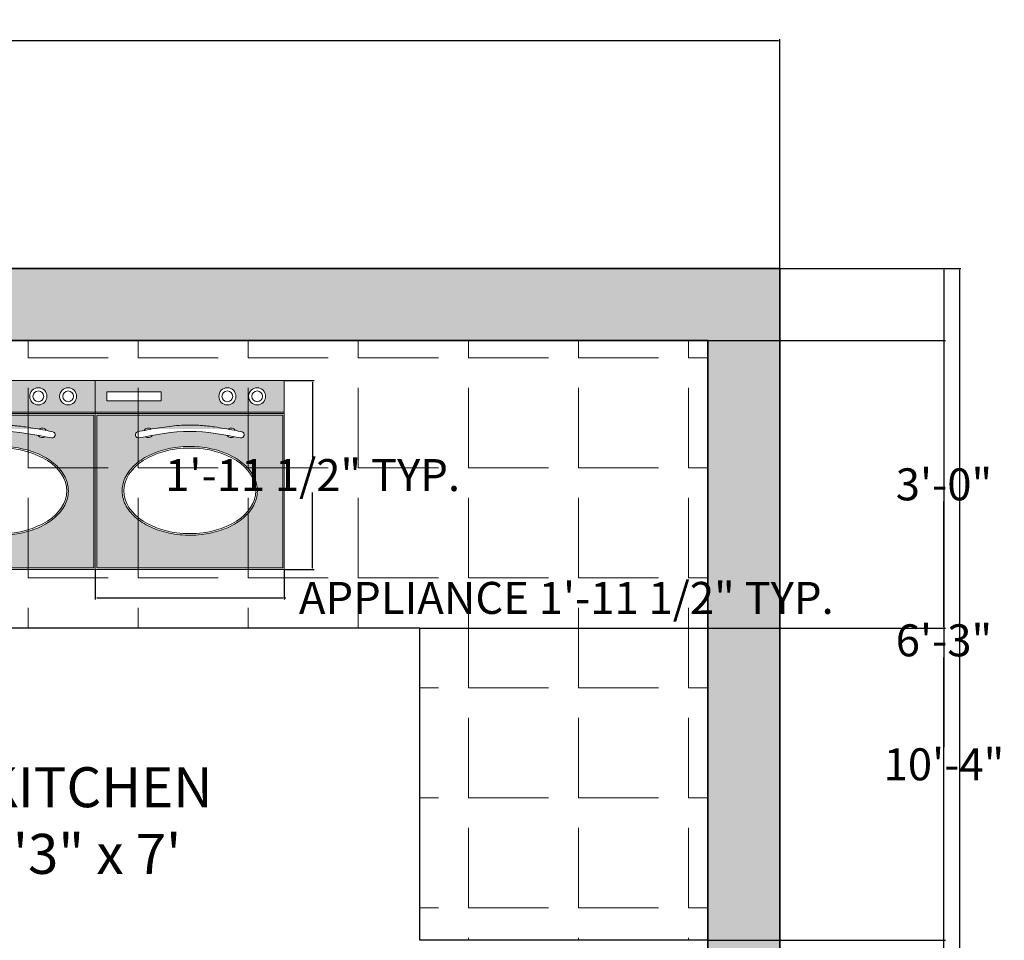
# Model space of a CAD drawing. Units: inches. Extents: x 490 to 851, y 299 to 716.
# Tile 3 of 3: x 728 to 851, y 601 to 716. Entities that reach past the tile are written whole.
import ezdxf

# ---------------------------------------------------------------- set-up
doc = ezdxf.new("R2010")
doc.units = ezdxf.units.IN
doc.header["$MEASUREMENT"] = 0
for name, color, linetype, lineweight in [('A-ANNO-DIMS', 2, 'Continuous', 18), ('A-AREA-IDEN', 7, 'Continuous', 25), ('A-EQPM', 8, 'Continuous', 18), ('A-EQPM-PATT', 9, 'Continuous', 13), ('A-FLOR-CASE', 40, 'Continuous', 25), ('A-FLOR-CASE-PATT', 9, 'Continuous', 13), ('A-WALL', 7, 'Continuous', 35), ('A-WALL-PATT', 1, 'Continuous', 13)]:
    doc.layers.add(name, color=color, linetype=linetype, lineweight=lineweight)
doc.styles.get("Standard").update_dxf_attribs({"font": 'arial.ttf'})
doc.dimstyles.get("Standard").update_dxf_attribs({"dimtxt": 4, "dimasz": 0.18, "dimexe": 0.18, "dimexo": 0.0625, "dimgap": 0.09, "dimtad": 0, "dimtih": 1, "dimtoh": 1, "dimdec": 0, "dimrnd": 6, "dimzin": 0, "dimdsep": 46, "dimlunit": 3, "dimtxsty": 'Standard', "dimcen": 0.09, "dimadec": 0, "dimazin": 0, "dimtfac": 1, "dimtdec": 0, "dimtofl": 0, "dimtmove": 0, "dimatfit": 3, "dimfxl": 1, "dimtolj": 1, "dimtzin": 0, "dimarcsym": 0})

# ---------------------------------------------------------------- blocks, each defined once
blk = doc.blocks.new('A$C7E884C79')
for p, q in [((-1.70119819813e-05, 1.5003966837e-05), (-1.70119419636e-05, 600.0000150039222)), ((-1.70119419636e-05, 600.0000150039222), (-1.70119819813e-05, 1.5003966837e-05)), ((-1.70119419636e-05, 600.0000150039222), (599.9999829879742, 600.0000150039077)), ((599.9999829879742, 600.0000150039077), (599.9999829880543, 1.5003966837e-05)), ((599.9999829880543, 1.5003966837e-05), (599.9999829879742, 600.0000150039077)), ((599.9999829879742, 600.0000150039077), (599.9999829879742, 450.0000150039659)), ((599.9999829879742, 600.0000150039077), (599.999982988058, 500.0000150039222)), ((599.999982988058, 500.0000150039222), (-1.70119383256e-05, 500.0000150039368)), ((599.999982988058, 495.0000150039441), (-1.70119019458e-05, 495.0000150039368)), ((599.999982988058, 500.0000150039222), (599.9999829880543, 1.5003966837e-05)), ((-1.70119819813e-05, 1.5003966837e-05), (599.9999829880543, 1.5003966837e-05))]:
    blk.add_line(p, q)
for points in [[(36.4219297853997, 564.739244228137), (208.9464086602384, 564.7392442281297), (208.9464086601583, 535.2607857798894), (36.4219297853997, 535.2607857798894)], [(4.999982988054398, 490.0000150040023), (594.999982988018, 490.0000150039513), (594.999982988018, 5.000015003966836), (4.999982987974362, 5.000015003930457)]]:
    blk.add_lwpolyline(points, close=True)
for centre, radius in [((419.341129777058, 550.0000150039514), 27.0465612830012), ((419.341129777058, 550.0000150039514), 17.0465612830012), ((513.9038640534054, 550.0000150040095), 27.0465612830012), ((513.9038640534054, 550.0000150040095), 17.0465612830012)]:
    blk.add_circle(centre, radius)
for centre, radius, start, end in [((168.4662399462322, 434.1738953022822), 14.99999999999999, 50.78880560725227, 150.3670062790382), ((431.5337276184946, 434.1738953023768), 14.99999999999999, 29.63299372096182, 129.2111943927477), ((137.2371143128039, 427.9571012842962), 9.99999999999936, 107.9829144627732, 276.9581094476087), ((168.4662399462322, 434.1738953022822), 14.99999999999999, 234.0164507050499, 327.1412143486447), ((431.5337276184946, 434.1738953023768), 14.99999999999999, 212.858785649389, 305.9835492949501), ((462.7628532516318, 427.957101284347), 9.99999999999936, 263.0418905523912, 72.01708553722673)]:
    blk.add_arc(centre, radius, start, end)
blk.add_ellipse((299.9999829880799, 250.0000150039296), major_axis=(-209.5453259160858, -5.8e-15), ratio=0.6483519184224599)
for points, knots in [([(134.1497789577479, 437.4685875095702), (144.6082166758169, 439.5062024863827), (155.1126203912208, 441.5529426086532), (185.9929094715517, 447.3437385568786), (206.494733029569, 450.9047119657725), (247.8674864836758, 456.3761860351832), (268.7408772092858, 458.286932131693), (293.5357101192494, 458.8504522635657), (297.2767330304487, 458.8901691064702), (304.7624299796444, 458.8727062536881), (308.4995762127364, 458.8160495901202), (319.6935092446511, 458.5127217792715), (327.132745431325, 458.1327232394569), (349.3790513168205, 456.541815341955), (364.1144689435605, 454.8805655177448), (399.790008761498, 449.8898845417889), (420.6328031065277, 446.1500348981672), (449.5099892856014, 440.6522069539087), (457.6940766911502, 439.0576405788188), (465.8501870183317, 437.4685875095119)], [0, 0, 0, 0, 31.63886493985545, 31.63886493985545, 92.6001428223882, 92.6001428223882, 153.561420704921, 153.561420704921, 164.3676472469802, 164.3676472469802, 175.1738737890395, 175.1738737890395, 196.786326873158, 196.786326873158, 240.011233041395, 240.011233041395, 302.0992006983722, 302.0992006983722, 326.7730650015291, 326.7730650015291, 326.7730650015291, 326.7730650015291]), ([(85.4546570720122, 250.000015003995), (85.45465707196854, 244.8170777658043), (85.88822561246344, 239.6342308201456), (88.02000493869853, 226.9220552357911), (90.21816192173355, 219.4365483580441), (96.38934370677816, 204.8396118246929), (100.3615888692657, 197.7281744404427), (109.949488846185, 184.0573372099134), (115.5648436689007, 177.4976038454224), (128.2787075515953, 165.0792487628459), (135.3771921305961, 159.2204529245464), (150.8720546014374, 148.3331296320939), (159.2684172301451, 143.3046103743872), (177.1485118738346, 134.1894280664528), (186.6321541176294, 130.1028504448732), (206.452394453896, 122.9637707452166), (216.7888352855625, 119.9113613978661), (238.0601333966843, 114.9105694415302), (248.9947899629697, 112.9622577759255), (271.1933164569673, 110.2148003270667), (282.4569621843111, 109.4156943254311), (305.0360465127196, 108.9852871540024), (316.3512522399324, 109.3539922337331), (338.7547296880475, 111.250649079022), (349.842772469201, 112.7785733309465), (371.5188673051307, 116.9582324470866), (382.1067079762179, 119.6099073260157), (402.521673323441, 125.9760737243086), (412.3486219806691, 129.6904786132982), (430.9992961862953, 138.0977836687561), (439.8229044345789, 142.7905902191232), (456.2471036538445, 153.0498538677457), (463.8476543751239, 158.616262825697), (477.6310685340795, 170.4997415048819), (483.8139313680366, 176.8169072710916), (494.5927765360757, 190.0604633081639), (499.1886010545786, 196.9871541335851), (506.6510537532812, 211.2839776396031), (509.5170666792983, 218.6543269104914), (513.4150547302415, 233.6388937332849), (514.4461961801352, 241.2525613148282), (514.6307693529524, 256.4928783461756), (513.7841458961847, 264.1183282945521), (510.2477897096396, 279.1482905806288), (507.5588601688614, 286.5521574531694), (500.4381704066108, 300.9341605102481), (496.0070741749878, 307.9124682590946), (485.5423204980033, 321.2743467604842), (479.5088542609591, 327.6582316730155), (466.0064121881987, 339.6881924907093), (458.5374402723464, 345.3343844510992), (442.356079099205, 355.7645443168249), (433.643722825036, 360.5484732858849), (415.1928234087136, 369.1474950443399), (405.4543904653837, 372.9624956318466), (385.1916535080673, 379.5371793190816), (374.6675208302404, 382.2967738713005), (353.0924824455687, 386.6971874674664), (342.0417855184496, 388.3379435140769), (319.6857084956864, 390.4625844960347), (308.380556257187, 390.9464386215868), (285.7940339416527, 390.7459687177425), (274.5128969021971, 390.0616475992965), (252.2522801997875, 387.5407311810659), (241.273026189534, 385.704172406523), (219.886530266871, 380.921302532438), (209.4794921704815, 377.9750595404139), (189.4937597145654, 371.0403800096638), (179.9152279588161, 367.0520348783057), (161.8232383307077, 358.1233102125143), (153.3098778178173, 353.1830191051149), (137.5613657555441, 342.4603322407738), (130.3262354594117, 336.6779568452357), (117.3219427482508, 324.3988645588861), (111.5527951950935, 317.9019950986867), (101.6427302403026, 304.3410831906103), (97.50207040229724, 297.2767107389691), (90.98281377420064, 282.7548846949166), (88.60495846102276, 275.2973569409469), (86.02335275324731, 261.8687924363285), (85.45465707200856, 255.934491795876), (85.4546570720122, 250.000015003995)], [0, 0, 0, 0, 0.1083005230516948, 0.1083005230516948, 0.2675342177864238, 0.2675342177864238, 0.4267679125211527, 0.4267679125211527, 0.5860016072558816, 0.5860016072558816, 0.7452353019906105, 0.7452353019906105, 0.9044689967253393, 0.9044689967253393, 1.063702691460068, 1.063702691460068, 1.222936386194797, 1.222936386194797, 1.382170080929526, 1.382170080929526, 1.541403775664254, 1.541403775664254, 1.700637470398983, 1.700637470398983, 1.859871165133712, 1.859871165133712, 2.019104859868441, 2.019104859868441, 2.17833855460317, 2.17833855460317, 2.337572249337898, 2.337572249337898, 2.496805944072627, 2.496805944072627, 2.656039638807356, 2.656039638807356, 2.815273333542085, 2.815273333542085, 2.974507028276814, 2.974507028276814, 3.133740723011543, 3.133740723011543, 3.292974417746271, 3.292974417746271, 3.452208112481, 3.452208112481, 3.611441807215729, 3.611441807215729, 3.770675501950458, 3.770675501950458, 3.929909196685187, 3.929909196685187, 4.089142891419916, 4.089142891419916, 4.248376586154645, 4.248376586154645, 4.407610280889374, 4.407610280889374, 4.566843975624102, 4.566843975624102, 4.726077670358831, 4.726077670358831, 4.88531136509356, 4.88531136509356, 5.044545059828289, 5.044545059828289, 5.203778754563018, 5.203778754563018, 5.363012449297746, 5.363012449297746, 5.522246144032475, 5.522246144032475, 5.681479838767204, 5.681479838767204, 5.840713533501933, 5.840713533501933, 5.999947228236662, 5.999947228236662, 6.15918092297139, 6.15918092297139, 6.283185307179586, 6.283185307179586, 6.283185307179586, 6.283185307179586])]:
    blk.add_open_spline(points, degree=3, knots=knots)
blk.add_open_spline([(137.9744605147498, 417.8376983042863), (191.9829680058602, 428.3601631990827), (299.999982988136, 449.4050929886863), (408.016997970407, 428.360163199051), (462.0255054615699, 417.837698304228)], degree=3)
blk = doc.blocks.new('*D102')
at = {"layer": 'A-ANNO-DIMS', "color": 0, "lineweight": -2, "transparency": 16777216}
for p, q in [((546.6878542437281, 685.0194991519433), (546.6878542437281, 713.5977998437985)), ((546.867854243728, 713.4177998437985), (681.1694777089394, 713.4177998437985)), ((822.507854243728, 713.4177998437985), (688.2062307785166, 713.4177998437985)), ((822.687854243728, 685.0194991519433), (822.687854243728, 713.5977998437985))]:
    blk.add_line(p, q, dxfattribs=at)
at = {"layer": 'A-ANNO-DIMS', "color": 0, "transparency": 16777216}
for points in [[(546.867854243728, 713.4477998437985), (546.867854243728, 713.3877998437985), (546.6878542437281, 713.4177998437985)], [(822.507854243728, 713.4477998437985), (822.507854243728, 713.3877998437985), (822.687854243728, 713.4177998437985)]]:
    blk.add_solid(points, dxfattribs=at)
at = {"layer": 'Defpoints', "color": 0, "transparency": 16777216}
for p in [(822.687854243728, 713.4177998437985), (546.6878542437281, 684.9569991519433), (822.687854243728, 684.9569991519433)]:
    blk.add_point(p, dxfattribs=at)
at = {"layer": 'A-ANNO-DIMS', "color": 0, "transparency": 16777216, "insert": (684.687854243728, 713.4177998437985), "char_height": 4, "attachment_point": 5}
blk.add_mtext("\\A1;23'", dxfattribs=at)
blk = doc.blocks.new('*D103')
at = {"layer": 'A-ANNO-DIMS', "color": 0, "lineweight": -2, "transparency": 16777216}
for p, q in [((822.7503542437285, 684.9569991519436), (845.3273379142681, 684.9569991519436)), ((845.147337914268, 684.7769991519436), (845.147337914268, 507.0906553593105)), ((845.147337914268, 325.1369991519435), (845.147337914268, 502.8233429445765)), ((822.7503542437283, 324.9569991519435), (845.3273379142681, 324.9569991519435))]:
    blk.add_line(p, q, dxfattribs=at)
at = {"layer": 'A-ANNO-DIMS', "color": 0, "transparency": 16777216}
for points in [[(845.117337914268, 684.7769991519436), (845.1773379142682, 684.7769991519436), (845.147337914268, 684.9569991519436)], [(845.117337914268, 325.1369991519435), (845.1773379142682, 325.1369991519435), (845.147337914268, 324.9569991519435)]]:
    blk.add_solid(points, dxfattribs=at)
at = {"layer": 'Defpoints', "color": 0, "transparency": 16777216}
for p in [(822.6878542437285, 684.9569991519436), (822.6878542437283, 324.9569991519435), (845.147337914268, 324.9569991519435)]:
    blk.add_point(p, dxfattribs=at)
at = {"layer": 'A-ANNO-DIMS', "color": 0, "transparency": 16777216, "insert": (845.147337914268, 504.9569991519431), "char_height": 4, "attachment_point": 5}
blk.add_mtext("\\A1;30'", dxfattribs=at)
blk = doc.blocks.new('*D114')
at = {"layer": 'A-ANNO-DIMS', "color": 0, "lineweight": -2, "transparency": 16777216}
for p, q in [((737.131587064389, 647.2418630191439), (737.131587064389, 643.5810559325296)), ((760.753634308485, 647.2418630191439), (760.753634308485, 643.5810559325296)), ((737.3115870643888, 643.7610559325295), (760.5736343084851, 643.7610559325295)), ((760.753634308485, 643.7610559325295), (760.933634308485, 643.7610559325295))]:
    blk.add_line(p, q, dxfattribs=at)
at = {"layer": 'A-ANNO-DIMS', "color": 0, "transparency": 16777216}
for points in [[(737.3115870643888, 643.7910559325294), (737.3115870643888, 643.7310559325294), (737.131587064389, 643.7610559325295)], [(760.5736343084851, 643.7910559325294), (760.5736343084851, 643.7310559325294), (760.753634308485, 643.7610559325295)]]:
    blk.add_solid(points, dxfattribs=at)
at = {"layer": 'Defpoints', "color": 0, "transparency": 16777216}
for p in [(737.131587064389, 647.3043630191439), (760.753634308485, 647.3043630191439), (760.753634308485, 643.7610559325295)]:
    blk.add_point(p, dxfattribs=at)
at = {"layer": 'A-ANNO-DIMS', "color": 0, "transparency": 16777216, "insert": (796.004534717762, 643.7610559325295), "char_height": 4, "attachment_point": 5}
blk.add_mtext('\\A1;APPLIANCE 1\'-11 1/2" TYP.', dxfattribs=at)
blk = doc.blocks.new('*D115')
at = {"layer": 'A-ANNO-DIMS', "color": 0, "lineweight": -2, "transparency": 16777216}
for p, q in [((760.8161343084852, 670.9264102632369), (764.4769413950997, 670.9264102632369)), ((764.2969413950999, 670.746410263237), (764.2969413950999, 661.2735994652013)), ((764.2969413950999, 647.4843630191441), (764.2969413950999, 656.9571738171796)), ((760.8161343084852, 647.3043630191441), (764.4769413950997, 647.3043630191441))]:
    blk.add_line(p, q, dxfattribs=at)
at = {"layer": 'A-ANNO-DIMS', "color": 0, "transparency": 16777216}
for points in [[(764.2669413950999, 670.746410263237), (764.3269413950998, 670.746410263237), (764.2969413950999, 670.9264102632369)], [(764.2669413950999, 647.4843630191441), (764.3269413950998, 647.4843630191441), (764.2969413950999, 647.3043630191441)]]:
    blk.add_solid(points, dxfattribs=at)
at = {"layer": 'Defpoints', "color": 0, "transparency": 16777216}
for p in [(760.7536343084852, 670.9264102632369), (764.2969413950999, 670.9264102632369), (760.7536343084852, 647.3043630191441)]:
    blk.add_point(p, dxfattribs=at)
at = {"layer": 'A-ANNO-DIMS', "color": 0, "transparency": 16777216, "insert": (764.2969413950999, 659.1153866411903), "char_height": 4, "attachment_point": 5}
blk.add_mtext('\\A1;1\'-11 1/2" TYP.', dxfattribs=at)
blk = doc.blocks.new('*D139')
at = {"layer": 'A-ANNO-DIMS', "color": 0, "lineweight": -2, "transparency": 16777216}
for p, q in [((813.7503540000004, 675.9569990000002), (843.3817780000008, 675.9569990000002)), ((843.2017780000009, 675.7769990000002), (843.2017780000009, 660.0906552073673)), ((843.2017780000009, 640.1369990000001), (843.2017780000009, 655.8233427926332)), ((777.7503540000004, 639.9569990000002), (843.3817780000008, 639.9569990000002))]:
    blk.add_line(p, q, dxfattribs=at)
at = {"layer": 'A-ANNO-DIMS', "color": 0, "transparency": 16777216}
for points in [[(843.171778000001, 675.7769990000002), (843.2317780000008, 675.7769990000002), (843.2017780000009, 675.9569990000002)], [(843.171778000001, 640.1369990000001), (843.2317780000008, 640.1369990000001), (843.2017780000009, 639.9569990000002)]]:
    blk.add_solid(points, dxfattribs=at)
at = {"layer": 'Defpoints', "color": 0, "transparency": 16777216}
for p in [(813.6878540000004, 675.9569990000002), (843.2017780000009, 675.9569990000002), (777.6878540000004, 639.9569990000002)]:
    blk.add_point(p, dxfattribs=at)
at = {"layer": 'A-ANNO-DIMS', "color": 0, "transparency": 16777216, "insert": (843.2017780000007, 657.9569989999998), "char_height": 4, "attachment_point": 5}
blk.add_mtext('\\A1;3\'-0"', dxfattribs=at)
blk = doc.blocks.new('*D140')
at = {"layer": 'A-ANNO-DIMS', "color": 0, "lineweight": -2, "transparency": 16777216}
for p, q in [((813.7503540000004, 675.9569990000002), (843.3817780000008, 675.9569990000002)), ((843.2017780000009, 675.7769990000002), (843.2017780000009, 640.5906552073671)), ((843.2017780000009, 601.1369990000002), (843.2017780000009, 636.3233427926331)), ((813.7503540000004, 600.9569990000002), (843.3817780000008, 600.9569990000002))]:
    blk.add_line(p, q, dxfattribs=at)
at = {"layer": 'A-ANNO-DIMS', "color": 0, "transparency": 16777216}
for points in [[(843.171778000001, 675.7769990000002), (843.2317780000008, 675.7769990000002), (843.2017780000009, 675.9569990000002)], [(843.171778000001, 601.1369990000002), (843.2317780000008, 601.1369990000002), (843.2017780000009, 600.9569990000002)]]:
    blk.add_solid(points, dxfattribs=at)
at = {"layer": 'Defpoints', "color": 0, "transparency": 16777216}
for p in [(813.6878540000004, 675.9569990000002), (843.2017780000009, 675.9569990000002), (813.6878540000004, 600.9569990000002)]:
    blk.add_point(p, dxfattribs=at)
at = {"layer": 'A-ANNO-DIMS', "color": 0, "transparency": 16777216, "insert": (843.2017780000007, 638.4569989999999), "char_height": 4, "attachment_point": 5}
blk.add_mtext('\\A1;6\'-3"', dxfattribs=at)
blk = doc.blocks.new('*D142')
at = {"layer": 'A-ANNO-DIMS', "color": 0, "lineweight": -2, "transparency": 16777216}
for p, q in [((822.7503540000004, 684.9569990000002), (843.3817780000008, 684.9569990000002)), ((843.2017780000009, 684.7769990000003), (843.2017780000009, 625.089290950887)), ((843.2017780000009, 561.1369990000001), (843.2017780000009, 620.8247070491134)), ((813.7503540000004, 560.9569990000002), (843.3817780000008, 560.9569990000002))]:
    blk.add_line(p, q, dxfattribs=at)
at = {"layer": 'A-ANNO-DIMS', "color": 0, "transparency": 16777216}
for points in [[(843.171778000001, 684.7769990000003), (843.2317780000008, 684.7769990000003), (843.2017780000009, 684.9569990000002)], [(843.171778000001, 561.1369990000001), (843.2317780000008, 561.1369990000001), (843.2017780000009, 560.9569990000002)]]:
    blk.add_solid(points, dxfattribs=at)
at = {"layer": 'Defpoints', "color": 0, "transparency": 16777216}
for p in [(822.6878540000004, 684.9569990000002), (843.2017780000009, 684.9569990000002), (813.6878540000004, 560.9569990000002)]:
    blk.add_point(p, dxfattribs=at)
at = {"layer": 'A-ANNO-DIMS', "color": 0, "transparency": 16777216, "insert": (843.2017780000007, 622.9569989999999), "char_height": 4, "attachment_point": 5}
blk.add_mtext('\\A1;10\'-4"', dxfattribs=at)

msp = doc.modelspace()

# ---------------------------------------------------------------- hatches: boundary and pattern name
at = {"layer": 'A-EQPM-PATT'}
h = msp.add_hatch(color=256, dxfattribs=at)
h.dxf.hatch_style = 1
edge = h.paths.add_edge_path(flags=0)
edge.add_ellipse((725.3205634423474, 657.1468827041818), major_axis=(8.249815980948258, 3.137e-13), ratio=0.648351918422466, start_angle=0, end_angle=360)
edge = h.paths.add_edge_path(flags=0)
edge.add_ellipse((748.9426106864386, 657.1468827041818), major_axis=(8.249815980948258, 3.137e-13), ratio=0.648351918422466, start_angle=0, end_angle=360)
h.paths.add_polyline_path([(760.5567839147827, 666.5957016018205), (737.3284374580912, 666.5957016018225), (737.328437458088, 647.5012134128433), (760.5567839147827, 647.5012134128445)])
edge = h.paths.add_edge_path(flags=16)
edge.add_spline(control_points=[(740.4959443117903, 657.1468827041843), (740.4959443117887, 656.9428300570115), (740.513013939367, 656.7387809646627), (740.5969422592976, 656.238301610948), (740.683483872803, 655.943596615761), (740.9264437855999, 655.368914075078), (741.0828313904223, 655.0889362253043), (741.4603077674664, 654.5507142870945), (741.6813847289907, 654.2924570680201), (742.181930551144, 653.8035454505958), (742.461398447955, 653.5728841971194), (743.0714324035, 653.1442494218261), (743.4019978613231, 652.9462762227037), (744.1059385953266, 652.5874107775095), (744.4793103372083, 652.4265218947702), (745.259634759896, 652.1454557648624), (745.6665812493317, 652.0252821685099), (746.5040339308719, 651.8284005954259), (746.934532220883, 651.7516954117406), (747.8084899568673, 651.6435277956438), (748.251940576054, 651.6120669294378), (749.1408809039442, 651.5951217652083), (749.5863614443855, 651.6096377132291), (750.4683881155711, 651.6843092425713), (750.9049252329394, 651.7444637406785), (751.758314793409, 651.9090172491879), (752.1751589143181, 652.0134138979646), (752.9788977075159, 652.2640503703385), (753.3657854499264, 652.4102867832906), (754.1000639619589, 652.7412830453165), (754.4474501134661, 652.926039208717), (755.0940721299727, 653.3299472263792), (755.393306410338, 653.5490971853537), (755.9359605110842, 654.0169506766601), (756.1793803076966, 654.2656579902905), (756.6037442906904, 654.7870578342696), (756.7846822638598, 655.0597621974754), (757.0784796142024, 655.6226292646414), (757.1913147687701, 655.9128004957787), (757.344778865264, 656.5027440714792), (757.3853749853384, 656.802494763666), (757.3926416456854, 657.4025072452151), (757.3593100135294, 657.7027218101118), (757.2200833920119, 658.2944526087763), (757.1142200242647, 658.5859434305298), (756.8338779076405, 659.152164023328), (756.6594253000964, 659.4269005488733), (756.2474271238373, 659.9529587575895), (756.0098890830087, 660.204292809264), (755.4782968754197, 660.6779133138975), (755.1842428629845, 660.9002043359601), (754.5471813994751, 661.310840551146), (754.2041752469486, 661.4991842113454), (753.4777618841014, 661.8377283750641), (753.0943590123167, 661.987925248588), (752.2966134628161, 662.246771063046), (751.8822775306182, 662.3554165178577), (751.0328665705918, 662.5286611476281), (750.5977997624374, 662.5932578423766), (749.7176392497302, 662.6769051251308), (749.2725545159311, 662.6959545001525), (748.3833213539021, 662.6880619842531), (747.9391821003803, 662.6611202079364), (747.0627798680019, 662.5618715300532), (746.63052577311, 662.4895660664885), (745.7885377446587, 662.3012641029419), (745.378811835352, 662.1852702843584), (744.591971974883, 661.912251405195), (744.214864425444, 661.7552299433305), (743.5025813692192, 661.403705350189), (743.1674096954835, 661.2092057002914), (742.5473895355515, 660.7870526741362), (742.2625418860974, 660.5594000995088), (741.750561858099, 660.0759712693376), (741.5234300646675, 659.820189007125), (741.1332700270774, 659.2862948375157), (740.9702519232188, 659.0081699378447), (740.7135882764434, 658.4364445030395), (740.6199719255308, 658.1428410481587), (740.5183339055397, 657.6141574062448), (740.4959443117901, 657.3805235227624), (740.4959443117903, 657.1468827041843)], knot_values=[0, 0, 0, 0, 0.1083005230516948, 0.1083005230516948, 0.2675342177864238, 0.2675342177864238, 0.4267679125211527, 0.4267679125211527, 0.5860016072558816, 0.5860016072558816, 0.7452353019906105, 0.7452353019906105, 0.9044689967253393, 0.9044689967253393, 1.063702691460068, 1.063702691460068, 1.222936386194797, 1.222936386194797, 1.382170080929526, 1.382170080929526, 1.541403775664254, 1.541403775664254, 1.700637470398983, 1.700637470398983, 1.859871165133712, 1.859871165133712, 2.019104859868441, 2.019104859868441, 2.17833855460317, 2.17833855460317, 2.337572249337898, 2.337572249337898, 2.496805944072627, 2.496805944072627, 2.656039638807356, 2.656039638807356, 2.815273333542085, 2.815273333542085, 2.974507028276814, 2.974507028276814, 3.133740723011543, 3.133740723011543, 3.292974417746271, 3.292974417746271, 3.452208112481, 3.452208112481, 3.611441807215729, 3.611441807215729, 3.770675501950458, 3.770675501950458, 3.929909196685187, 3.929909196685187, 4.089142891419916, 4.089142891419916, 4.248376586154645, 4.248376586154645, 4.407610280889374, 4.407610280889374, 4.566843975624102, 4.566843975624102, 4.726077670358831, 4.726077670358831, 4.88531136509356, 4.88531136509356, 5.044545059828289, 5.044545059828289, 5.203778754563018, 5.203778754563018, 5.363012449297746, 5.363012449297746, 5.522246144032475, 5.522246144032475, 5.681479838767204, 5.681479838767204, 5.840713533501933, 5.840713533501933, 5.999947228236662, 5.999947228236662, 6.15918092297139, 6.15918092297139, 6.283185307179586, 6.283185307179586, 6.283185307179586, 6.283185307179586], degree=3, periodic=0)
edge = h.paths.add_edge_path(flags=0)
edge.add_ellipse((748.9426106864386, 657.1468827041818), major_axis=(8.249815980948258, 3.137e-13), ratio=0.648351918422466, start_angle=0, end_angle=360)
edge = h.paths.add_edge_path(flags=16)
edge.add_spline(control_points=[(742.4130750946933, 664.5275351650338), (742.6914882918603, 664.5817783431816), (742.9707288907302, 664.6361857766777), (743.2508036674241, 664.6898164654069)], knot_values=[0, 0, 0, 0, 21.39329177210675, 21.39329177210675, 21.39329177210675, 21.39329177210675], degree=3, periodic=0)
edge.add_arc((743.7641168658934, 664.3978228734082), 0.5905511811023694, 50.78880560234279, 150.3670062825767, ccw=False)
edge.add_spline(control_points=[(744.1374519240431, 664.8553943233596), (744.779067646516, 664.97139206178), (745.4250780596886, 665.0781755879807), (746.8901501941393, 665.2719288077744), (747.7119372305805, 665.3471550320465), (748.688111754595, 665.36934086401), (748.8353961211775, 665.3709045192425), (749.1301085994924, 665.3702170053534), (749.2772403409527, 665.3679864280476), (749.7179463658312, 665.3560443882504), (750.0108296802672, 665.3410838158167), (750.8866684946568, 665.2784496466238), (751.4668030468905, 665.2130461102375), (752.8713518586205, 665.0165626072471), (753.6919343131492, 664.8693244323014), (754.8288314068135, 664.6528745132362), (755.1510395723863, 664.5900963094923), (755.4721462781808, 664.5275351650314)], knot_values=[43.89785635095746, 43.89785635095746, 43.89785635095746, 43.89785635095746, 92.6001428223882, 92.6001428223882, 153.561420704921, 153.561420704921, 164.3676472469802, 164.3676472469802, 175.1738737890395, 175.1738737890395, 196.786326873158, 196.786326873158, 240.011233041395, 240.011233041395, 302.0992006983722, 302.0992006983722, 326.7730650015291, 326.7730650015291, 326.7730650015291, 326.7730650015291], degree=3, periodic=0)
edge.add_arc((754.1211045695258, 664.397822873412), 0.5905511811023695, 29.64555569566221, 129.3131094229314, ccw=False)
edge.add_spline(control_points=[(744.1374519240431, 664.8553943233596), (744.779067646516, 664.97139206178), (745.4250780596886, 665.0781755879807), (746.8901501941393, 665.2719288077744), (747.7119372305805, 665.3471550320465), (748.688111754595, 665.36934086401), (748.8353961211775, 665.3709045192425), (749.1301085994924, 665.3702170053534), (749.2772403409527, 665.3679864280476), (749.7179463658312, 665.3560443882504), (750.0108296802672, 665.3410838158167), (750.8866684946568, 665.2784496466238), (751.4668030468905, 665.2130461102375), (752.8713518586205, 665.0165626072471), (753.6919343131492, 664.8693244323014), (754.8288314068135, 664.6528745132362), (755.1510395723863, 664.5900963094923), (755.4721462781808, 664.5275351650314)], knot_values=[43.89785635095746, 43.89785635095746, 43.89785635095746, 43.89785635095746, 92.6001428223882, 92.6001428223882, 153.561420704921, 153.561420704921, 164.3676472469802, 164.3676472469802, 175.1738737890395, 175.1738737890395, 196.786326873158, 196.786326873158, 240.011233041395, 240.011233041395, 302.0992006983722, 302.0992006983722, 326.7730650015291, 326.7730650015291, 326.7730650015291, 326.7730650015291], degree=3, periodic=0)
edge.add_arc((755.3505977046888, 664.1530672034108), 0.3937007874015679, -101.0087676412142, 72.01708553236932, ccw=False)
edge.add_spline(control_points=[(755.3215682641351, 663.7546655112802), (755.037073723253, 663.810093516205), (754.7525791823709, 663.8655215211298), (754.4680846414888, 663.9199572781217)], knot_values=[304.9124823041715, 304.9124823041715, 304.9124823041715, 304.9124823041715, 326.7730650015789, 326.7730650015789, 326.7730650015789, 326.7730650015789], degree=3, periodic=0)
edge.add_arc((754.1211045695258, 664.397822873412), 0.5905511811023683, 212.8587871331284, 305.9835477310444, ccw=False)
edge.add_spline(control_points=[(753.6250354635439, 664.0774073001456), (752.0642272045088, 664.3599897262603), (748.9426107100477, 664.8064223787223), (745.8209942155868, 664.3599897330135), (744.2601859801605, 664.0774073129695)], knot_values=[43.45390602737222, 43.45390602737222, 43.45390602737222, 43.45390602737222, 163.3865343148396, 283.3191607881738, 283.3191607881738, 283.3191607881738, 283.3191607881738], degree=3, periodic=0)
edge.add_arc((743.7641168658934, 664.3978228734082), 0.5905511811023553, 234.01645070441748, 327.1412143484826, ccw=False)
edge.add_spline(control_points=[(743.417136780882, 663.9199572875928), (743.1326422235041, 663.8655215275596), (742.8481476661264, 663.8100935194209), (742.5636531087486, 663.7546655112824)], knot_values=[0, 0, 0, 0, 21.86058396493695, 21.86058396493695, 21.86058396493695, 21.86058396493695], degree=3, periodic=0)
edge.add_arc((742.5346237307191, 664.1530672034088), 0.393700787401568, 107.9829001472302, 281.00876763934195, ccw=False)
h.paths.add_polyline_path([(736.9347366706914, 666.5957016018205), (713.706390214, 666.5957016018225), (713.7063902139969, 647.5012134128433), (736.9347366706914, 647.5012134128445)])
edge = h.paths.add_edge_path(flags=16)
edge.add_spline(control_points=[(716.8738970676992, 657.1468827041843), (716.8738970676975, 656.9428300570115), (716.8909666952759, 656.7387809646627), (716.9748950152064, 656.238301610948), (717.0614366287118, 655.943596615761), (717.3043965415088, 655.368914075078), (717.4607841463312, 655.0889362253043), (717.8382605233752, 654.5507142870945), (718.0593374848995, 654.2924570680201), (718.5598833070528, 653.8035454505958), (718.8393512038638, 653.5728841971194), (719.4493851594088, 653.1442494218261), (719.7799506172319, 652.9462762227037), (720.4838913512355, 652.5874107775095), (720.8572630931171, 652.4265218947702), (721.6375875158049, 652.1454557648624), (722.0445340052405, 652.0252821685099), (722.8819866867807, 651.8284005954259), (723.312484976792, 651.7516954117406), (724.1864427127762, 651.6435277956438), (724.6298933319629, 651.6120669294378), (725.518833659853, 651.5951217652083), (725.9643142002944, 651.6096377132291), (726.84634087148, 651.6843092425713), (727.2828779888483, 651.7444637406785), (728.136267549318, 651.9090172491879), (728.5531116702269, 652.0134138979646), (729.3568504634247, 652.2640503703385), (729.7437382058351, 652.4102867832906), (730.4780167178678, 652.7412830453165), (730.825402869375, 652.926039208717), (731.4720248858815, 653.3299472263792), (731.7712591662468, 653.5490971853537), (732.3139132669932, 654.0169506766601), (732.5573330636055, 654.2656579902905), (732.9816970465993, 654.7870578342696), (733.1626350197686, 655.0597621974754), (733.4564323701113, 655.6226292646414), (733.5692675246789, 655.9128004957787), (733.7227316211728, 656.5027440714792), (733.7633277412472, 656.802494763666), (733.7705944015944, 657.4025072452151), (733.7372627694382, 657.7027218101118), (733.5980361479207, 658.2944526087763), (733.4921727801734, 658.5859434305298), (733.2118306635494, 659.152164023328), (733.0373780560052, 659.4269005488733), (732.6253798797461, 659.9529587575895), (732.3878418389176, 660.204292809264), (731.8562496313285, 660.6779133138975), (731.5621956188934, 660.9002043359601), (730.925134155384, 661.310840551146), (730.5821280028575, 661.4991842113454), (729.8557146400102, 661.8377283750641), (729.4723117682256, 661.987925248588), (728.6745662187249, 662.246771063046), (728.2602302865271, 662.3554165178577), (727.4108193265005, 662.5286611476281), (726.9757525183463, 662.5932578423766), (726.0955920056391, 662.6769051251308), (725.65050727184, 662.6959545001525), (724.761274109811, 662.6880619842531), (724.317134856289, 662.6611202079364), (723.4407326239107, 662.5618715300532), (723.0084785290189, 662.4895660664885), (722.1664905005676, 662.3012641029419), (721.7567645912609, 662.1852702843584), (720.9699247307918, 661.912251405195), (720.5928171813528, 661.7552299433305), (719.880534125128, 661.403705350189), (719.5453624513922, 661.2092057002914), (718.9253422914603, 660.7870526741362), (718.6404946420062, 660.5594000995088), (718.1285146140078, 660.0759712693376), (717.9013828205763, 659.820189007125), (717.5112227829862, 659.2862948375157), (717.3482046791275, 659.0081699378447), (717.0915410323522, 658.4364445030395), (716.9979246814397, 658.1428410481587), (716.8962866614485, 657.6141574062448), (716.8738970676989, 657.3805235227624), (716.8738970676992, 657.1468827041843)], knot_values=[0, 0, 0, 0, 0.1083005230516948, 0.1083005230516948, 0.2675342177864238, 0.2675342177864238, 0.4267679125211527, 0.4267679125211527, 0.5860016072558816, 0.5860016072558816, 0.7452353019906105, 0.7452353019906105, 0.9044689967253393, 0.9044689967253393, 1.063702691460068, 1.063702691460068, 1.222936386194797, 1.222936386194797, 1.382170080929526, 1.382170080929526, 1.541403775664254, 1.541403775664254, 1.700637470398983, 1.700637470398983, 1.859871165133712, 1.859871165133712, 2.019104859868441, 2.019104859868441, 2.17833855460317, 2.17833855460317, 2.337572249337898, 2.337572249337898, 2.496805944072627, 2.496805944072627, 2.656039638807356, 2.656039638807356, 2.815273333542085, 2.815273333542085, 2.974507028276814, 2.974507028276814, 3.133740723011543, 3.133740723011543, 3.292974417746271, 3.292974417746271, 3.452208112481, 3.452208112481, 3.611441807215729, 3.611441807215729, 3.770675501950458, 3.770675501950458, 3.929909196685187, 3.929909196685187, 4.089142891419916, 4.089142891419916, 4.248376586154645, 4.248376586154645, 4.407610280889374, 4.407610280889374, 4.566843975624102, 4.566843975624102, 4.726077670358831, 4.726077670358831, 4.88531136509356, 4.88531136509356, 5.044545059828289, 5.044545059828289, 5.203778754563018, 5.203778754563018, 5.363012449297746, 5.363012449297746, 5.522246144032475, 5.522246144032475, 5.681479838767204, 5.681479838767204, 5.840713533501933, 5.840713533501933, 5.999947228236662, 5.999947228236662, 6.15918092297139, 6.15918092297139, 6.283185307179586, 6.283185307179586, 6.283185307179586, 6.283185307179586], degree=3, periodic=0)
edge = h.paths.add_edge_path(flags=0)
edge.add_ellipse((725.3205634423474, 657.1468827041818), major_axis=(8.249815980948258, 3.137e-13), ratio=0.648351918422466, start_angle=0, end_angle=360)
edge = h.paths.add_edge_path(flags=16)
edge.add_spline(control_points=[(731.6995210200438, 663.7546655112802), (731.4150264791617, 663.810093516205), (731.1305319382795, 663.8655215211298), (730.8460373973976, 663.9199572781217)], knot_values=[304.9124823041715, 304.9124823041715, 304.9124823041715, 304.9124823041715, 326.7730650015789, 326.7730650015789, 326.7730650015789, 326.7730650015789], degree=3, periodic=0)
edge.add_arc((730.4990573254347, 664.397822873412), 0.5905511811023683, 212.8587871331377, 305.9835477310444, ccw=False)
edge.add_spline(control_points=[(730.0029882194526, 664.0774073001456), (728.4421799604175, 664.3599897262603), (725.3205634659566, 664.8064223787223), (722.1989469714956, 664.3599897330135), (720.6381387360695, 664.0774073129695)], knot_values=[43.45390602737222, 43.45390602737222, 43.45390602737222, 43.45390602737222, 163.3865343148396, 283.3191607881738, 283.3191607881738, 283.3191607881738, 283.3191607881738], degree=3, periodic=0)
edge.add_arc((720.1420696218023, 664.3978228734082), 0.5905511811023554, 234.01645070441748, 327.14121434847334, ccw=False)
edge.add_spline(control_points=[(719.7950895367909, 663.9199572875928), (719.5105949794131, 663.8655215275596), (719.2261004220353, 663.8100935194209), (718.9416058646574, 663.7546655112824)], knot_values=[0, 0, 0, 0, 21.86058396493695, 21.86058396493695, 21.86058396493695, 21.86058396493695], degree=3, periodic=0)
edge.add_arc((718.9125764866279, 664.1530672034088), 0.393700787401568, 107.9829001472302, 281.00876763934195, ccw=False)
edge.add_spline(control_points=[(718.7910278506022, 664.5275351650338), (719.0694410477691, 664.5817783431816), (719.3486816466392, 664.6361857766777), (719.628756423333, 664.6898164654069)], knot_values=[0, 0, 0, 0, 21.39329177210675, 21.39329177210675, 21.39329177210675, 21.39329177210675], degree=3, periodic=0)
edge.add_arc((720.1420696218023, 664.3978228734082), 0.5905511811023695, 50.78880560234978, 150.3670062825767, ccw=False)
edge.add_spline(control_points=[(720.5154046799519, 664.8553943233596), (721.1570204024248, 664.97139206178), (721.8030308155975, 665.0781755879807), (723.268102950048, 665.2719288077744), (724.0898899864894, 665.3471550320465), (725.0660645105037, 665.36934086401), (725.2133488770864, 665.3709045192425), (725.5080613554012, 665.3702170053534), (725.6551930968615, 665.3679864280476), (726.0958991217401, 665.3560443882504), (726.388782436176, 665.3410838158167), (727.2646212505655, 665.2784496466238), (727.8447558027995, 665.2130461102375), (729.2493046145294, 665.0165626072471), (730.069887069058, 664.8693244323014), (731.2067841627223, 664.6528745132362), (731.5289923282951, 664.5900963094923), (731.8500990340896, 664.5275351650314)], knot_values=[43.89785635095746, 43.89785635095746, 43.89785635095746, 43.89785635095746, 92.6001428223882, 92.6001428223882, 153.561420704921, 153.561420704921, 164.3676472469802, 164.3676472469802, 175.1738737890395, 175.1738737890395, 196.786326873158, 196.786326873158, 240.011233041395, 240.011233041395, 302.0992006983722, 302.0992006983722, 326.7730650015291, 326.7730650015291, 326.7730650015291, 326.7730650015291], degree=3, periodic=0)
edge.add_arc((730.4990573254347, 664.397822873412), 0.5905511811023695, 29.64555569566221, 129.3131094229314, ccw=False)
edge.add_spline(control_points=[(720.5154046799519, 664.8553943233596), (721.1570204024248, 664.97139206178), (721.8030308155975, 665.0781755879807), (723.268102950048, 665.2719288077744), (724.0898899864894, 665.3471550320465), (725.0660645105037, 665.36934086401), (725.2133488770864, 665.3709045192425), (725.5080613554012, 665.3702170053534), (725.6551930968615, 665.3679864280476), (726.0958991217401, 665.3560443882504), (726.388782436176, 665.3410838158167), (727.2646212505655, 665.2784496466238), (727.8447558027995, 665.2130461102375), (729.2493046145294, 665.0165626072471), (730.069887069058, 664.8693244323014), (731.2067841627223, 664.6528745132362), (731.5289923282951, 664.5900963094923), (731.8500990340896, 664.5275351650314)], knot_values=[43.89785635095746, 43.89785635095746, 43.89785635095746, 43.89785635095746, 92.6001428223882, 92.6001428223882, 153.561420704921, 153.561420704921, 164.3676472469802, 164.3676472469802, 175.1738737890395, 175.1738737890395, 196.786326873158, 196.786326873158, 240.011233041395, 240.011233041395, 302.0992006983722, 302.0992006983722, 326.7730650015291, 326.7730650015291, 326.7730650015291, 326.7730650015291], degree=3, periodic=0)
edge.add_arc((731.7285504605976, 664.1530672034108), 0.393700787401568, -101.0087676412142, 72.01708553236932, ccw=False)
h.paths.add_polyline_path([(737.1315870643906, 670.9264102632361), (713.5095398202994, 670.9264102632366), (713.5095398202992, 666.9894023892214), (737.131587064391, 666.9894023892209)])
h.paths.add_polyline_path([(728.954208541008, 668.9579063262299, -1), (731.0838590357325, 668.9579063262299, -1)], flags=16)
h.paths.add_polyline_path([(729.3479093284096, 668.9579063262299, -1), (730.6901582483309, 668.9579063262299, -1)], flags=0)
h.paths.add_polyline_path([(721.7357770514844, 668.3776217111093), (714.9434747335805, 668.3776217111093), (714.9434747335805, 669.5381909413553), (721.7357770514876, 669.538190941355)], flags=16)
h.paths.add_polyline_path([(732.6771508353524, 668.9579063262321, -1), (734.806801330077, 668.9579063262321, -1)], flags=16)
h.paths.add_polyline_path([(733.070851622754, 668.9579063262321, -1), (734.4131005426754, 668.9579063262321, -1)], flags=0)
h.paths.add_polyline_path([(760.7536343084817, 670.9264102632361), (737.1315870643906, 670.9264102632366), (737.131587064391, 666.9894023892214), (760.7536343084823, 666.9894023892209)])
h.paths.add_polyline_path([(752.5762557850992, 668.9579063262299, -1), (754.7059062798236, 668.9579063262299, -1)], flags=16)
h.paths.add_polyline_path([(745.3578242955756, 668.3776217111093), (738.5655219776717, 668.3776217111093), (738.5655219776717, 669.5381909413553), (745.3578242955788, 669.538190941355)], flags=16)
h.paths.add_polyline_path([(754.3122054924221, 668.9579063262299, -1), (752.9699565725008, 668.9579063262299, -1)], flags=0)
h.paths.add_polyline_path([(758.4288485741681, 668.9579063262321, -1), (756.2991980794436, 668.9579063262321, -1)], flags=16)
h.paths.add_polyline_path([(758.0351477867665, 668.9579063262321, -1), (756.6928988668451, 668.9579063262321, -1)], flags=0)
at = {"layer": 'A-FLOR-CASE-PATT'}
h = msp.add_hatch(dxfattribs=at)
h.set_pattern_fill('ANGLE', color=256, scale=50)
h.set_pattern_definition([(0, (0, 0), (0, 13.75), [10, -3.75]), (90, (0, 0), (-13.75, 8e-16), [10, -3.75])])
h.paths.add_polyline_path([(813.687854243728, 675.9569991519433), (691.6878542437281, 675.9569991519433), (691.6878542437281, 639.9569991519435), (777.6878542437281, 639.9569991519434), (777.6878542437279, 600.9569991519433), (813.6878542437278, 600.9569991519433)])
at = {"layer": 'A-WALL-PATT'}
h = msp.add_hatch(color=256, dxfattribs=at)
h.dxf.hatch_style = 1
h.paths.add_polyline_path([(555.6878542437281, 497.9569991519433), (611.6878542437282, 497.9569991519434), (611.6878542437281, 493.9569991519433), (615.6878542437281, 493.9569991519433), (615.6878542437281, 501.9569991519433), (555.6878542437281, 501.9569991519433), (555.6878542437281, 529.9569991519433), (651.6878542437281, 529.9569991519433), (651.6878542437281, 533.9569991519433), (555.6878542437281, 533.9569991519433), (555.6878542437281, 675.9569991519433), (813.687854243728, 675.9569991519433), (813.6878542437278, 564.9569991519431), (813.6878542437278, 560.9569991519431), (813.6878542437278, 533.9569991519433), (802.5034207310172, 533.9569991519433), (802.5034207310172, 529.9569991519433), (813.687854243728, 529.9569991519433), (813.687854243728, 465.9569991519433), (727.6878542437282, 465.9569991519433), (727.6878542437282, 461.9569991519433), (813.687854243728, 461.9569991519433), (813.687854243728, 333.9569991519434), (786.3863959033706, 333.9569991519434), (786.3863959033706, 324.9569991519434), (822.687854243728, 324.9569991519434), (822.687854243728, 684.9569991519433), (546.6878542437281, 684.9569991519433), (546.6878542437281, 324.9569991519434), (555.7079255371355, 324.9569991519434), (555.7079255371355, 333.9569991519433), (555.6878542437281, 333.9569991519433), (555.6878542437281, 461.9569991519433), (651.6878542437282, 461.9569991519433), (651.6878542437282, 465.9569991519433), (555.6878542437281, 465.9569991519433)])
h.paths.add_polyline_path([(714.3863959033706, 333.9569991519433), (691.6878542437281, 333.9569991519433), (691.6878542437282, 429.9205150877742), (691.6792956389427, 429.9205150877742), (691.6792956389427, 465.9569991519433), (687.6878542437282, 465.9569991519433), (687.6878542437282, 429.9569991519434), (687.6878542437281, 361.0075905803756), (687.6936932778153, 361.0075905803756), (687.6936932778153, 324.9569991519434), (714.3863959033706, 324.9569991519434)], flags=17)
h.paths.add_polyline_path([(691.6878542437281, 675.9569991519433), (687.6878542437281, 675.9569991519433), (687.6878542437282, 529.9569991519433), (691.6878542437282, 529.9569991519433)], flags=17)
h.paths.add_polyline_path([(777.7575047331366, 533.9569991519433), (761.6878542437282, 533.9569991519433), (761.6878542437282, 497.9569991519433, -0.0312398925164955), (765.6878542437281, 498.2098446269331), (765.6878542437281, 529.9569991519433), (777.7575047331366, 529.9569991519433)], flags=17)
h.paths.add_polyline_path([(777.6878542437279, 564.9569991519434), (727.687854243728, 564.9569991519433), (727.687854243728, 560.9569991519434), (777.6878542437279, 560.9569991519434)], flags=17)

# ---------------------------------------------------------------- linework, layer by layer
at = {"layer": 'A-FLOR-CASE'}
for p, q in [((777.6878542437282, 639.9569991519434), (691.6878542437281, 639.9569991519435)), ((777.6878542437279, 600.9569991519433), (777.6878542437281, 639.9569991519435)), ((813.687854243728, 600.9569991519433), (777.6878542437281, 600.9569991519433))]:
    msp.add_line(p, q, dxfattribs=at)
at = {"layer": 'A-WALL'}
for p, q in [((822.687854243728, 684.9569991519433), (546.6878542437281, 684.9569991519433)), ((822.687854243728, 324.9569991519434), (822.687854243728, 684.9569991519433)), ((813.687854243728, 675.9569991519433), (555.6878542437281, 675.9569991519433)), ((813.6878542437278, 564.9569991519431), (813.687854243728, 675.9569991519433))]:
    msp.add_line(p, q, dxfattribs=at)

# ---------------------------------------------------------------- block references
at = {"layer": 'A-EQPM', "xscale": 0.0393700787401575, "yscale": 0.0393700787401575, "zscale": 0.0393700787401575}
for p in [(713.5095404900608, 647.3043624284365), (737.131587734152, 647.3043624284365)]:
    msp.add_blockref('A$C7E884C79', p, dxfattribs=at)

# ---------------------------------------------------------------- texts
at = {"layer": 'A-AREA-IDEN', "insert": (723.0449506801868, 622.59746330636), "char_height": 5, "attachment_point": 1}
msp.add_mtext_dynamic_manual_height_columns('KITCHEN\\P9\'3" x 7\'', width=54.99209744262703, gutter_width=1, heights=[0], dxfattribs=at)

# ---------------------------------------------------------------- dimensions: what is measured, and where the dimension line sits
at = {"layer": 'A-ANNO-DIMS'}
dim = msp.add_linear_dim(base=(822.687854243728, 713.4177998437985), p1=(546.6878542437281, 684.9569991519433), p2=(822.687854243728, 684.9569991519433), dimstyle='Standard', override={"dimclrd": 0, "dimclre": 0, "dimclrt": 0}, dxfattribs=at)
dim.commit()
dim.dimension.update_dxf_attribs({"geometry": '*D102', "text_midpoint": (684.687854243728, 713.4177998437985)})
for base, p1, p2, override, picture, middle in [((843.2017780000009, 684.9569990000002), (813.6878539999999, 560.9569989999999), (822.6878539999999, 684.9569989999999), {"dimdec": 1, "dimlfac": 1, "dimrnd": 0, "dimzin": 1, "dimdsep": 46, "dimlunit": 4, "dimfrac": 2}, '*D142', (843.2017780000007, 622.9569989999999)), ((845.147337914268, 324.9569991519435), (822.687854243728, 684.9569991519433), (822.6878542437278, 324.9569991519434), {"dimclrd": 0, "dimclre": 0, "dimclrt": 0}, '*D103', (845.147337914268, 504.9569991519431)), ((843.2017780000009, 675.9569990000002), (777.687854, 639.9569989999999), (813.6878539999999, 675.956999), {"dimdec": 1, "dimlfac": 1, "dimrnd": 0, "dimzin": 1, "dimdsep": 46, "dimlunit": 4, "dimfrac": 2}, '*D139', (843.2017780000007, 657.9569989999998)), ((843.2017780000009, 675.9569990000002), (813.6878539999999, 600.956999), (813.6878539999999, 675.956999), {"dimdec": 1, "dimlfac": 1, "dimrnd": 0, "dimzin": 1, "dimdsep": 46, "dimlunit": 4, "dimfrac": 2}, '*D140', (843.2017780000007, 638.4569989999999))]:
    dim = msp.add_linear_dim(base=base, p1=p1, p2=p2, angle=90, dimstyle='Standard', override=override, dxfattribs=at)
    dim.commit()
    dim.dimension.update_dxf_attribs({"geometry": picture, "text_midpoint": middle})
dim = msp.add_linear_dim(base=(764.2969413950999, 670.9264102632369), p1=(760.753634308485, 647.3043630191439), p2=(760.753634308485, 670.9264102632366), angle=90, text='<> TYP.', dimstyle='Standard', override={"dimdec": 1, "dimlfac": 1, "dimrnd": 0, "dimzin": 1, "dimdsep": 46, "dimlunit": 4, "dimfrac": 2}, dxfattribs=at)
dim.commit()
dim.dimension.update_dxf_attribs({"geometry": '*D115', "text_midpoint": (764.2969413950999, 659.1153866411903)})
dim = msp.add_linear_dim(base=(760.753634308485, 643.7610559325295), p1=(737.131587064389, 647.3043630191439), p2=(760.753634308485, 647.3043630191439), text='APPLIANCE <> TYP.', dimstyle='Standard', override={"dimdec": 1, "dimlfac": 1, "dimrnd": 0, "dimzin": 1, "dimdsep": 46, "dimlunit": 4, "dimfrac": 2}, dxfattribs=at)
dim.commit()
dim.dimension.update_dxf_attribs({"geometry": '*D114', "text_midpoint": (796.004534717762, 643.7610559325295)})

doc.saveas('drawing.dxf')
